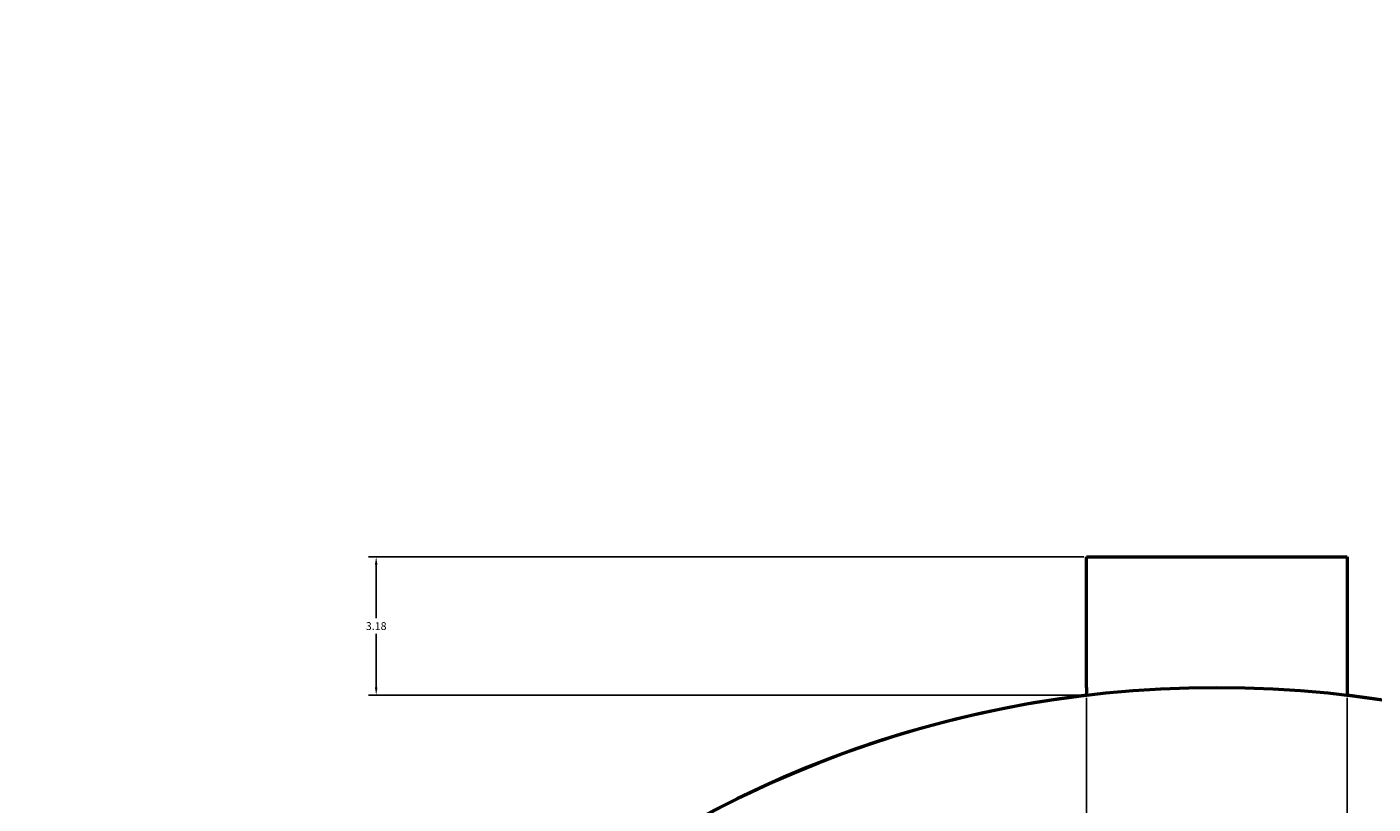
# Model space of a CAD drawing. Units: inches. Extents: x -99 to 284, y -92 to 134.
# Tile 5 of 16: x 5 to 36, y 37 to 55. Entities that reach past the tile are written whole.
import ezdxf

# ---------------------------------------------------------------- set-up
doc = ezdxf.new("R2010")
doc.units = ezdxf.units.IN
doc.header["$MEASUREMENT"] = 0
doc.layers.add('M-DIMS', color=2, linetype='Continuous', lineweight=18)
doc.layers.add('M-OUTL', color=7, linetype='Continuous', lineweight=50)
doc.styles.get("Standard").update_dxf_attribs({"font": 'arial.ttf'})
doc.dimstyles.get("Standard").update_dxf_attribs({"dimtxt": 0.18, "dimasz": 0.18, "dimexe": 0.18, "dimexo": 0.0625, "dimgap": 0.09, "dimtad": 0, "dimtih": 1, "dimtoh": 1, "dimdec": 4, "dimzin": 0, "dimdsep": 46, "dimtxsty": 'Standard', "dimcen": 0.09, "dimadec": 0, "dimazin": 0, "dimtfac": 1, "dimtdec": 4, "dimtofl": 0, "dimtmove": 0, "dimatfit": 3, "dimfxl": 1, "dimtolj": 1, "dimtzin": 0, "dimarcsym": 0})

# ---------------------------------------------------------------- blocks, each defined once
blk = doc.blocks.new('*D3')
at = {"layer": 'Defpoints', "color": 0, "transparency": 16777216}
for p in [(28.976, 39.673), (34.976, 39.673), (28.976, 23.323)]:
    blk.add_point(p, dxfattribs=at)
at = {"layer": 'M-DIMS', "color": 0, "lineweight": -2, "transparency": 16777216}
for p, q in [((28.976, 39.611), (28.976, 23.143)), ((34.976, 39.611), (34.976, 23.143)), ((29.156, 23.323), (31.827, 23.323)), ((34.796, 23.323), (32.126, 23.323))]:
    blk.add_line(p, q, dxfattribs=at)
at = {"layer": 'M-DIMS', "color": 0, "transparency": 16777216}
for points in [[(29.156, 23.353), (29.156, 23.293), (28.976, 23.323)], [(34.796, 23.353), (34.796, 23.293), (34.976, 23.323)]]:
    blk.add_solid(points, dxfattribs=at)
at = {"layer": 'M-DIMS', "color": 0, "transparency": 16777216, "insert": (31.976, 23.323), "char_height": 0.18, "attachment_point": 5}
blk.add_mtext('\\A1;6', dxfattribs=at)
blk = doc.blocks.new('*D4')
at = {"layer": 'Defpoints', "color": 0, "transparency": 16777216}
for p in [(12.626, 42.854), (28.976, 42.854), (28.976, 39.673)]:
    blk.add_point(p, dxfattribs=at)
at = {"layer": 'M-DIMS', "color": 0, "lineweight": -2, "transparency": 16777216}
for p, q in [((28.914, 42.854), (12.446, 42.854)), ((12.626, 42.674), (12.626, 41.446)), ((12.626, 39.853), (12.626, 41.082)), ((28.914, 39.673), (12.446, 39.673))]:
    blk.add_line(p, q, dxfattribs=at)
at = {"layer": 'M-DIMS', "color": 0, "transparency": 16777216}
for points in [[(12.596, 42.674), (12.656, 42.674), (12.626, 42.854)], [(12.596, 39.853), (12.656, 39.853), (12.626, 39.673)]]:
    blk.add_solid(points, dxfattribs=at)
at = {"layer": 'M-DIMS', "color": 0, "transparency": 16777216, "insert": (12.626, 41.264), "char_height": 0.18, "attachment_point": 5}
blk.add_mtext('\\A1;3.18', dxfattribs=at)
blk = doc.blocks.new('*D9')
at = {"layer": 'Defpoints', "color": 0, "transparency": 16777216}
for p in [(26.771, 58.303), (-73.374, 14.854), (31.976, 14.854)]:
    blk.add_point(p, dxfattribs=at)
at = {"layer": 'M-DIMS', "color": 0, "lineweight": -2, "transparency": 16777216}
for p, q in [((26.709, 58.303), (-73.554, 58.303)), ((-73.374, 58.123), (-73.374, 36.761)), ((-73.374, 15.034), (-73.374, 36.397)), ((31.914, 14.854), (-73.554, 14.854))]:
    blk.add_line(p, q, dxfattribs=at)
at = {"layer": 'M-DIMS', "color": 0, "transparency": 16777216}
for points in [[(-73.404, 58.123), (-73.344, 58.123), (-73.374, 58.303)], [(-73.404, 15.034), (-73.344, 15.034), (-73.374, 14.854)]]:
    blk.add_solid(points, dxfattribs=at)
at = {"layer": 'M-DIMS', "color": 0, "transparency": 16777216, "insert": (-73.374, 36.579), "char_height": 0.18, "attachment_point": 5}
blk.add_mtext('\\A1;43.45', dxfattribs=at)
blk = doc.blocks.new('*D19')
at = {"layer": 'Defpoints', "color": 0, "transparency": 16777216}
for p in [(112.982, 51.721), (-49.029, -22.013)]:
    blk.add_point(p, dxfattribs=at)
at = {"layer": 'M-DIMS', "color": 0, "lineweight": -2, "transparency": 16777216}
for p, q in [((31.976, 14.764), (31.976, 14.944)), ((31.886, 14.854), (32.066, 14.854)), ((-97.632, -44.133), (-49.192, -22.088)), ((-97.812, -44.133), (-97.632, -44.133))]:
    blk.add_line(p, q, dxfattribs=at)
at = {"layer": 'M-DIMS', "color": 0, "transparency": 16777216}
blk.add_solid([(-49.205, -22.06), (-49.18, -22.115), (-49.029, -22.013)], dxfattribs=at)
at = {"layer": 'M-DIMS', "color": 0, "transparency": 16777216, "insert": (-98.199, -44.133), "char_height": 0.18, "attachment_point": 5}
blk.add_mtext('\\A1;∅178', dxfattribs=at)
blk = doc.blocks.new('*D20')
at = {"layer": 'Defpoints', "color": 0, "transparency": 16777216}
for p in [(-35.23, 65.245), (99.183, -35.537)]:
    blk.add_point(p, dxfattribs=at)
at = {"layer": 'M-DIMS', "color": 0, "lineweight": -2, "transparency": 16777216}
for p, q in [((31.976, 14.764), (31.976, 14.944)), ((31.886, 14.854), (32.066, 14.854)), ((139.507, -65.772), (99.327, -35.645)), ((139.687, -65.772), (139.507, -65.772))]:
    blk.add_line(p, q, dxfattribs=at)
at = {"layer": 'M-DIMS', "color": 0, "transparency": 16777216}
blk.add_solid([(99.345, -35.621), (99.309, -35.669), (99.183, -35.537)], dxfattribs=at)
at = {"layer": 'M-DIMS', "color": 0, "transparency": 16777216, "insert": (140.074, -65.772), "char_height": 0.18, "attachment_point": 5}
blk.add_mtext('\\A1;∅168', dxfattribs=at)
blk = doc.blocks.new('*D22')
at = {"layer": 'Defpoints', "color": 0, "transparency": 16777216}
for p in [(39, 89.203), (31.976, 14.854)]:
    blk.add_point(p, dxfattribs=at)
at = {"layer": 'M-DIMS', "color": 0, "lineweight": -2, "transparency": 16777216}
for p, q in [((43.215, 133.813), (39.017, 89.383)), ((43.395, 133.813), (43.215, 133.813)), ((31.976, 14.764), (31.976, 14.944)), ((31.886, 14.854), (32.066, 14.854))]:
    blk.add_line(p, q, dxfattribs=at)
at = {"layer": 'M-DIMS', "color": 0, "transparency": 16777216}
blk.add_solid([(38.987, 89.385), (39.047, 89.38), (39, 89.203)], dxfattribs=at)
at = {"layer": 'M-DIMS', "color": 0, "transparency": 16777216, "insert": (44.068, 133.813), "char_height": 0.18, "attachment_point": 5}
blk.add_mtext('\\A1;5X R74.68', dxfattribs=at)

msp = doc.modelspace()

# ---------------------------------------------------------------- linework, layer by layer
at = {"layer": 'M-OUTL'}
for p, q in [((28.9765, 39.8539), (28.9765, 42.8539)), ((28.9765, 42.8539), (34.9765, 42.8539)), ((34.9765, 42.8539), (34.9765, 39.6732)), ((28.9765, 39.8539), (28.9765, 39.6732))]:
    msp.add_line(p, q, dxfattribs=at)
for radius in [89, 84, 25]:
    msp.add_circle((31.9765, 14.8539), radius, dxfattribs=at)
msp.add_arc((31.9765, 14.8539), 25, 96.8921, 83.1079, dxfattribs=at)

# ---------------------------------------------------------------- dimensions: what is measured, and where the dimension line sits
at = {"layer": 'M-DIMS'}
dim = msp.add_radius_dim(center=(31.9765, 14.8539), mpoint=(39.0003, 89.2035), text='5X <>', dimstyle='Standard', override={"dimdec": 2, "dimlfac": 1, "dimrnd": 0, "dimzin": 0, "dimdsep": 46, "dimlunit": 2}, dxfattribs=at)
dim.commit()
dim.dimension.update_dxf_attribs({"geometry": '*D22', "text_midpoint": (44.068, 133.8132), "dimtype": 164})
for p1, p2, picture, middle in [((-35.2301, 65.2451), (99.1831, -35.5373), '*D20', (140.074, -65.772)), ((112.9816, 51.7208), (-49.0286, -22.013), '*D19', (-98.1987, -44.1332))]:
    dim = msp.add_diameter_dim_2p(p1=p1, p2=p2, dimstyle='Standard', override={"dimdec": 0, "dimlfac": 1, "dimrnd": 0, "dimzin": 0, "dimdsep": 46, "dimlunit": 2}, dxfattribs=at)
    dim.commit()
    dim.dimension.update_dxf_attribs({"geometry": picture, "text_midpoint": middle, "dimtype": 163})
for base, p1, p2, angle, override, picture, middle in [((-73.3735, 14.8539), (26.7713, 58.3032), (31.9765, 14.8539), 90, {"dimdec": 2, "dimlfac": 1, "dimrnd": 0, "dimzin": 0, "dimdsep": 46, "dimlunit": 2}, '*D9', (-73.3735, 36.5785)), ((12.6265, 42.8539), (28.9765, 39.6732), (28.9765, 42.8539), 90, {"dimdec": 2, "dimlfac": 1, "dimrnd": 0, "dimzin": 0, "dimdsep": 46, "dimlunit": 2}, '*D4', (12.6265, 41.2636)), ((28.9765, 23.3232), (34.9765, 39.6732), (28.9765, 39.6732), 180, {"dimdec": 0, "dimlfac": 1, "dimrnd": 0, "dimzin": 0, "dimdsep": 46, "dimlunit": 2}, '*D3', (31.9765, 23.3232))]:
    dim = msp.add_linear_dim(base=base, p1=p1, p2=p2, angle=angle, dimstyle='Standard', override=override, dxfattribs=at)
    dim.commit()
    dim.dimension.update_dxf_attribs({"geometry": picture, "text_midpoint": middle})

doc.saveas('drawing.dxf')
